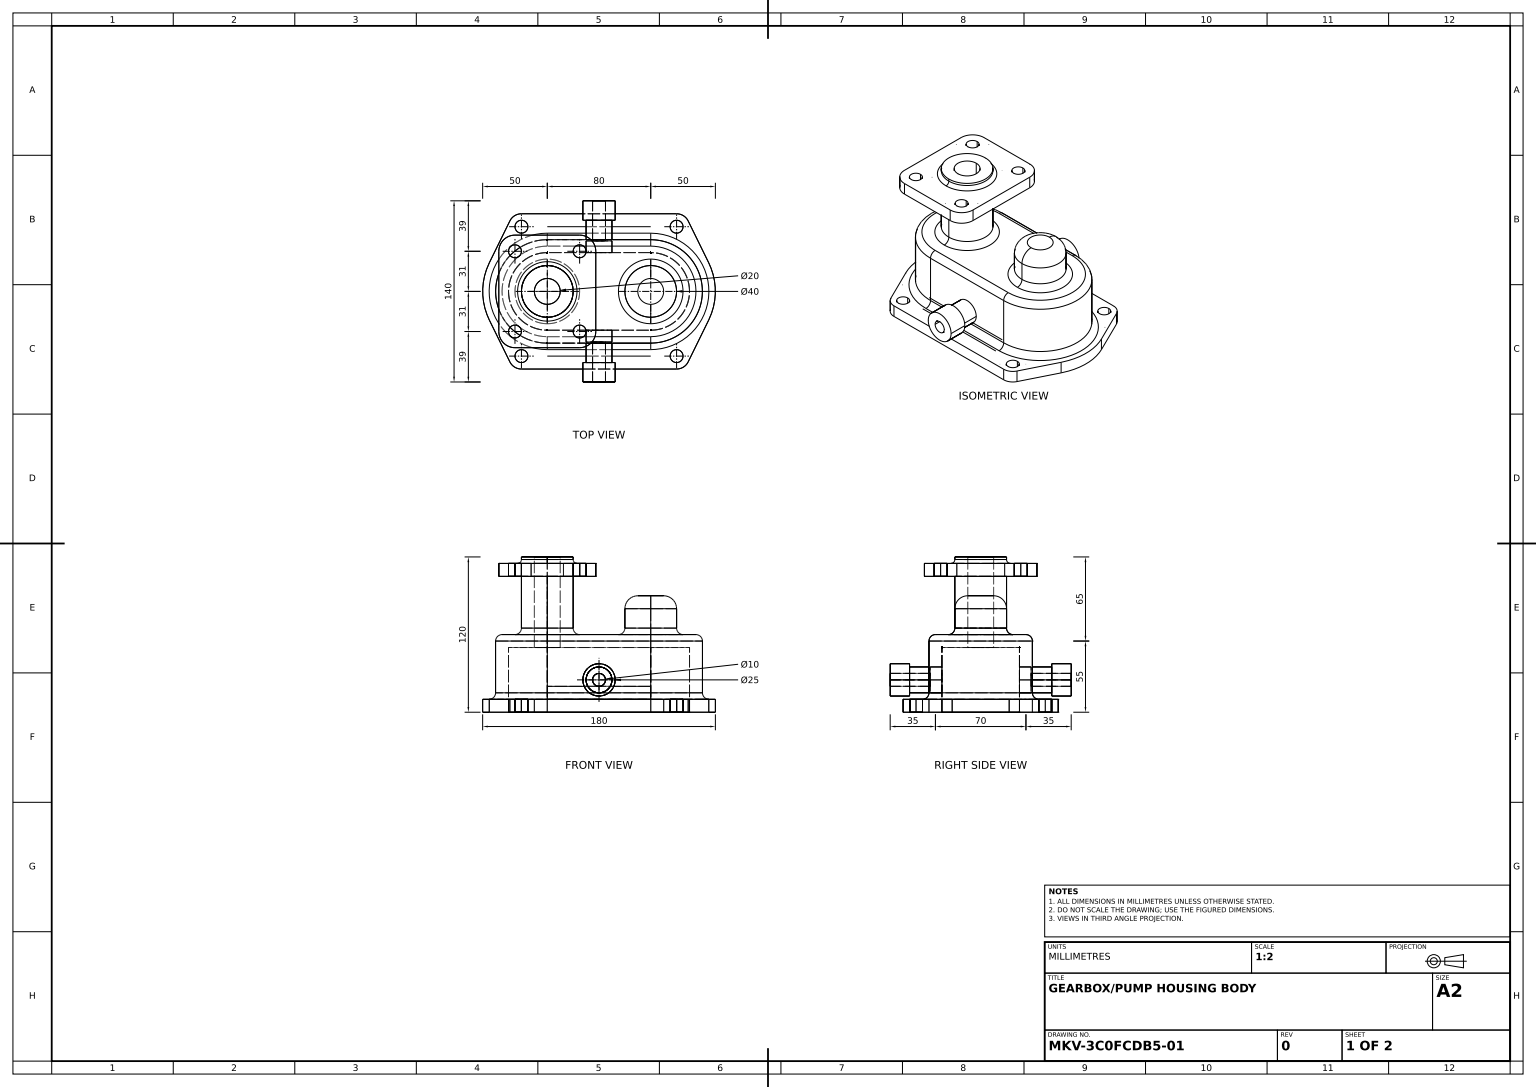
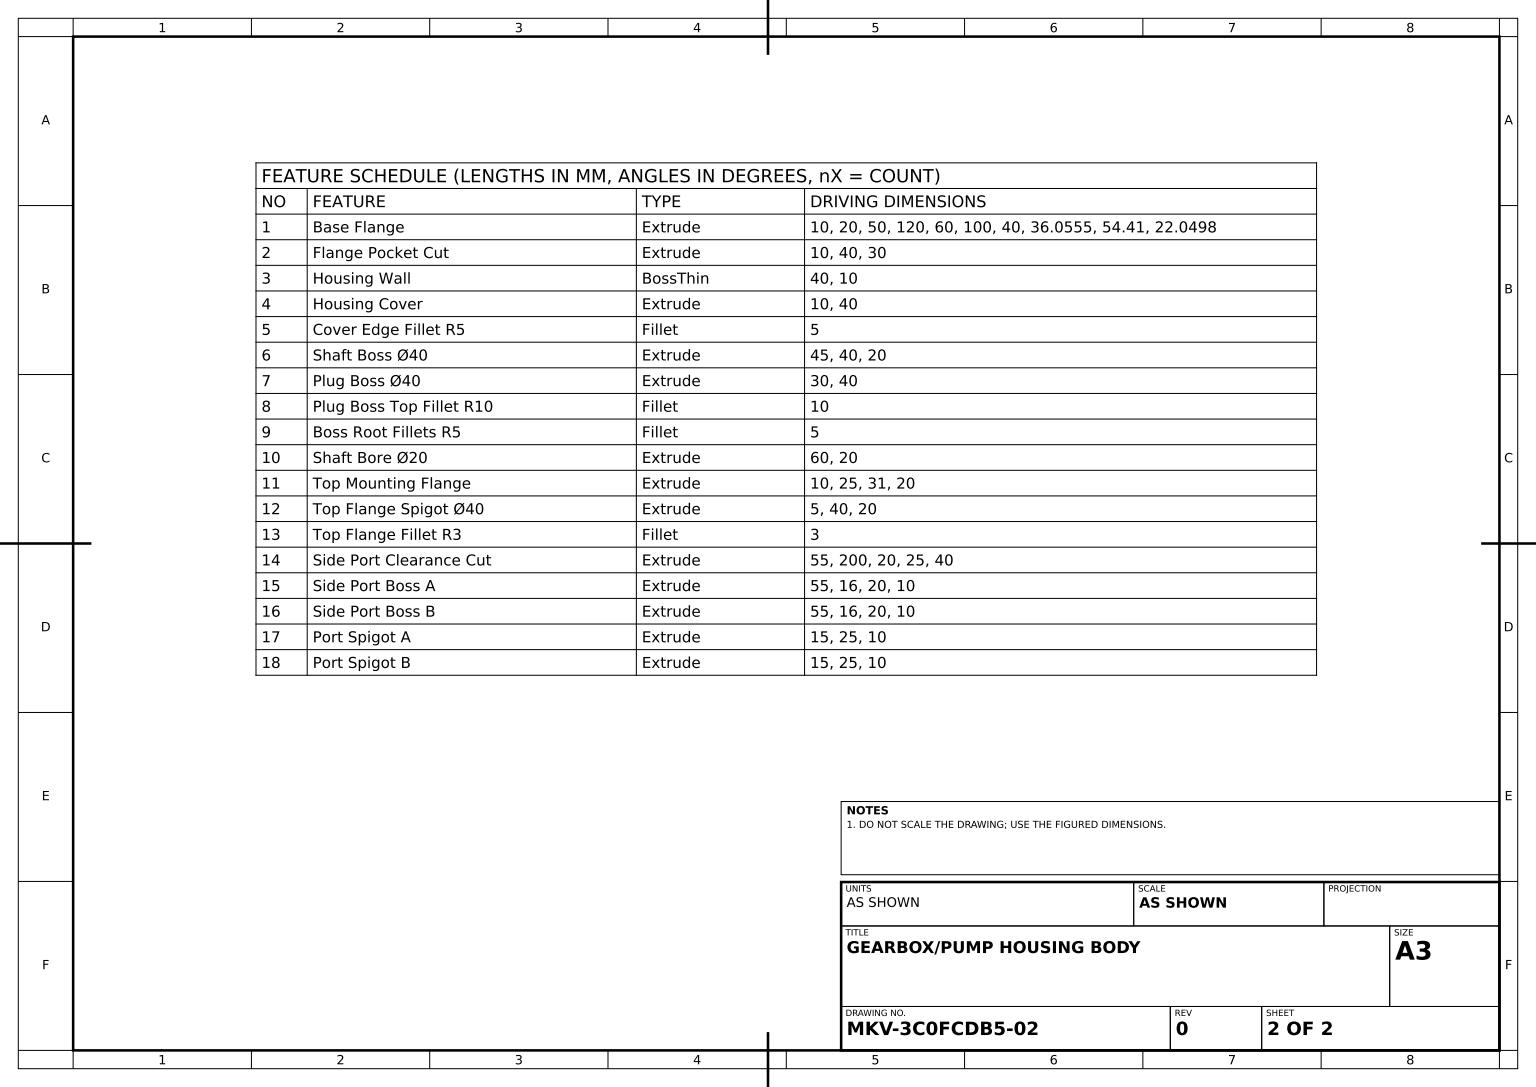
SolidWorks part; units mm, degrees
material "Plain Carbon Steel"
ref_plane "Front Plane" through (0, 0, 0) normal (0, 0, 1) x (1, 0, 0)
ref_plane "Top Plane" through (0, 0, 0) normal (0, 1, 0) x (1, 0, 0)
ref_plane "Right Plane" through (0, 0, 0) normal (1, 0, 0) x (0, 0, -1)
sketch "Base Flange Sketch" plane through (0, 0, 0) normal (0, 1, 0) x (1, 0, 0)
  line L0 (-60, 60) -> (60, 60)
  line L1 (-60, -60) -> (60, -60)
  line L2 (-84.8754, 22.0498) -> (-68.9751, 54.41)
  line L3 (-84.8754, -22.0498) -> (-68.9751, -54.41)
  line L4 (84.8754, 22.0498) -> (68.9751, 54.41)
  line L5 (84.8754, -22.0498) -> (68.9751, -54.41)
  circle A0 centre (-60, 50) radius 5
  arc A1 (-60, 60) -> (-68.9751, 54.41) centre (-60, 50) ccw
  circle A2 centre (-60, -50) radius 5
  arc A3 (-68.9751, -54.41) -> (-60, -60) centre (-60, -50) ccw
  circle A4 centre (60, 50) radius 5
  arc A5 (68.9751, 54.41) -> (60, 60) centre (60, 50) ccw
  circle A6 centre (60, -50) radius 5
  arc A7 (60, -60) -> (68.9751, -54.41) centre (60, -50) ccw
  arc A8 (-84.8754, 22.0498) -> (-84.8754, -22.0498) centre (-40, 0) ccw
  arc A10 (84.8754, -22.0498) -> (84.8754, 22.0498) centre (40, 0) ccw
  dimension "D1" = 20
  dimension "D2" = 10
  dimension "D3" = 36.0555
  dimension "D4" = 10
  dimension "D5" = 54.41
  dimension "D6" = 10
  dimension "D7" = 20
  dimension "D8" = 10
  dimension "D15" = 60
  dimension "D19" = 100
  dimension "D20" = 22.0498
  dimension "D22" = 40
  dimension "D9" = 50
  dimension "D10" = 50
  dimension "D11" = 50
  dimension "D12" = 50
  dimension "D13" = 120
  dimension "D14" = 60
  dimension "D16" = 120
  dimension "D17" = 120
  dimension "D18" = 120
  dimension "D21" = 40
  dimension "D23" = 60
  dimension "D24" = 60
extrude "Base Flange" add sketch "Base Flange Sketch" along normal blind 10
sketch "Flange Pocket Sketch" plane through (0, 10, 0) normal (0, 1, 0) x (1, 0, 0)
  line L1 (-40, 0) -> (40, 0) construction
  line L2 (-40, 30) -> (40, 30)
  line L3 (-40, -30) -> (40, -30)
  arc A0 (-40, 30) -> (-40, -30) centre (-40, 0) ccw
  arc A1 (40, -30) -> (40, 30) centre (40, 0) ccw
  point P0 (0, 0)
  point P4 (0, 0)
  dimension "D2" = 30
  dimension "D1" = 40
extrude "Flange Pocket Cut" cut sketch "Flange Pocket Sketch" against normal blind 10
sketch "Housing Wall Sketch" plane through (0, 10, 0) normal (0, 1, 0) x (1, 0, 0)
  line L0 (-40, 0) -> (40, 0) construction
  line L1 (-40, 40) -> (40, 40)
  line L2 (-40, -40) -> (40, -40)
  arc A0 (-40, 40) -> (-40, -40) centre (-40, 0) ccw
  arc A1 (40, -40) -> (40, 40) centre (40, 0) ccw
  point P4 (0, 0)
  dimension "D1" = 40
extrude "Housing Wall" add sketch "Housing Wall Sketch" along normal blind 40 thin
sketch "Housing Cover Sketch" plane through (0, 50, 0) normal (0, 1, 0) x (1, 0, 0)
  line L0 (-40, 0) -> (40, 0) construction
  line L1 (-40, 40) -> (40, 40)
  line L2 (-40, -40) -> (40, -40)
  arc A0 (-40, 40) -> (-40, -40) centre (-40, 0) ccw
  arc A1 (40, -40) -> (40, 40) centre (40, 0) ccw
  point P4 (0, 0)
  dimension "D1" = 40
extrude "Housing Cover" add sketch "Housing Cover Sketch" along normal blind 10
fillet "Cover Edge Fillet R5" radius 5 8 edges at (-80, 10, 0) (0, 10, 40) (80, 10, 0) (0, 10, -40) (-80, 60, 0) (0, 60, 40) (80, 60, 0) (0, 60, -40)
sketch "Shaft Boss Sketch" plane through (0, 60, 0) normal (0, 1, 0) x (1, 0, 0)
  circle A0 centre (-40, 0) radius 20
  circle A1 centre (-40, 0) radius 10
  dimension "D1" = 40
  dimension "D2" = 20
extrude "Shaft Boss Ø40" add sketch "Shaft Boss Sketch" along normal blind 45
sketch "Plug Boss Sketch" plane through (0, 60, 0) normal (0, 1, 0) x (1, 0, 0)
  circle A0 centre (40, 0) radius 20
  dimension "D1" = 40
extrude "Plug Boss Ø40" add sketch "Plug Boss Sketch" along normal blind 30
fillet "Plug Boss Top Fillet R10" radius 10 1 edges at (40, 90, 20)
fillet "Boss Root Fillets R5" radius 5 2 edges at (40, 60, 20) (-40, 60, 20)
sketch "Shaft Bore Sketch" plane through (0, 105, 0) normal (0, 1, 0) x (1, 0, 0)
  circle A0 centre (-40, 0) radius 10
  dimension "D1" = 20
extrude "Shaft Bore Ø20" cut sketch "Shaft Bore Sketch" against normal blind 60
sketch "Top Mounting Flange Sketch" plane through (0, 105, 0) normal (0, 1, 0) x (1, 0, 0)
  line L1 (-65, 43.5) -> (-15, 43.5)
  line L2 (-77.5, 31) -> (-77.5, -31)
  line L3 (-65, -43.5) -> (-15, -43.5)
  line L4 (-2.5, 31) -> (-2.5, -31)
  circle A0 centre (-65, 31) radius 5
  arc A1 (-65, 43.5) -> (-77.5, 31) centre (-65, 31) ccw
  circle A2 centre (-15, 31) radius 5
  arc A3 (-2.5, 31) -> (-15, 43.5) centre (-15, 31) ccw
  circle A4 centre (-65, -31) radius 5
  arc A5 (-77.5, -31) -> (-65, -43.5) centre (-65, -31) ccw
  circle A6 centre (-15, -31) radius 5
  arc A7 (-15, -43.5) -> (-2.5, -31) centre (-15, -31) ccw
  circle A9 centre (-40, 0) radius 10
  dimension "D1" = 25
  dimension "D2" = 25
  dimension "D3" = 10
  dimension "D4" = 10
  dimension "D5" = 10
  dimension "D6" = 25
  dimension "D7" = 10
  dimension "D8" = 25
  dimension "D17" = 20
  dimension "D9" = 25
  dimension "D10" = 25
  dimension "D11" = 25
  dimension "D12" = 25
  dimension "D13" = 31
  dimension "D14" = 31
  dimension "D15" = 31
  dimension "D16" = 31
extrude "Top Mounting Flange" add sketch "Top Mounting Flange Sketch" along normal blind 10
sketch "Top Flange Spigot Sketch" plane through (0, 115, 0) normal (0, 1, 0) x (1, 0, 0)
  circle A0 centre (-40, 0) radius 10
  circle A1 centre (-40, 0) radius 20
  dimension "D1" = 40
  dimension "D2" = 20
extrude "Top Flange Spigot Ø40" add sketch "Top Flange Spigot Sketch" along normal blind 5
fillet "Top Flange Fillet R3" radius 3 1 edges at (-40, 115, 20)
ref_plane "Plane1" through (0, 0, 55) normal (0, 0, 1) x (1, 0, 0)
sketch "Side Port Cut Sketch" plane through (0, 0, 55) normal (0, 0, 1) x (1, 0, 0)
  line L0 (-60, 0) -> (60, 0) construction
  line L1 (40, 55) -> (40, 15) construction
  circle A0 centre (0, 25) radius 10
  dimension "D1" = 20
  dimension "D3" = 25
  dimension "D4" = 40
extrude "Side Port Clearance Cut" cut sketch "Side Port Cut Sketch" against normal blind 200
sketch "Side Port Boss A Sketch" plane through (0, 0, 55) normal (0, 0, 1) x (1, 0, 0)
  circle A0 centre (0, 25) radius 10
  circle A1 centre (0, 25) radius 5
  dimension "D1" = 20
  dimension "D2" = 10
extrude "Side Port Boss A" add sketch "Side Port Boss A Sketch" against normal blind 16
ref_plane "Plane2" through (0, 0, -55) normal (0, 0, 1) x (1, 0, 0)
sketch "Side Port Boss B Sketch" plane through (0, 0, -55) normal (0, 0, 1) x (1, 0, 0)
  circle A0 centre (0, 25) radius 5
  circle A1 centre (0, 25) radius 10
  dimension "D1" = 20
  dimension "D2" = 10
extrude "Side Port Boss B" add sketch "Side Port Boss B Sketch" along normal blind 16
sketch "Port Spigot A Sketch" plane through (0, 0, 55) normal (0, 0, 1) x (1, 0, 0)
  circle A0 centre (0, 25) radius 12.5
  circle A1 centre (0, 25) radius 5
  dimension "D1" = 25
  dimension "D2" = 10
extrude "Port Spigot A" add sketch "Port Spigot A Sketch" along normal blind 15
sketch "Port Spigot B Sketch" plane through (0, 0, -55) normal (0, 0, -1) x (-1, 0, 0)
  circle A0 centre (0, 25) radius 5
  circle A1 centre (0, 25) radius 12.5
  dimension "D1" = 25
  dimension "D2" = 10
extrude "Port Spigot B" add sketch "Port Spigot B Sketch" along normal blind 15
